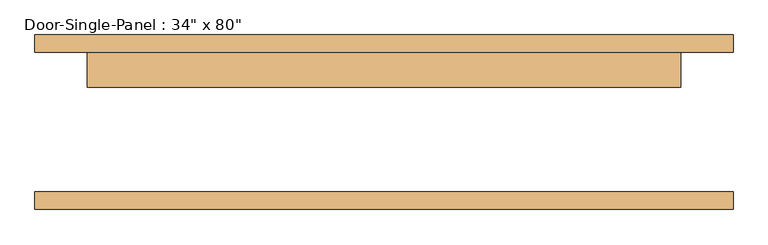
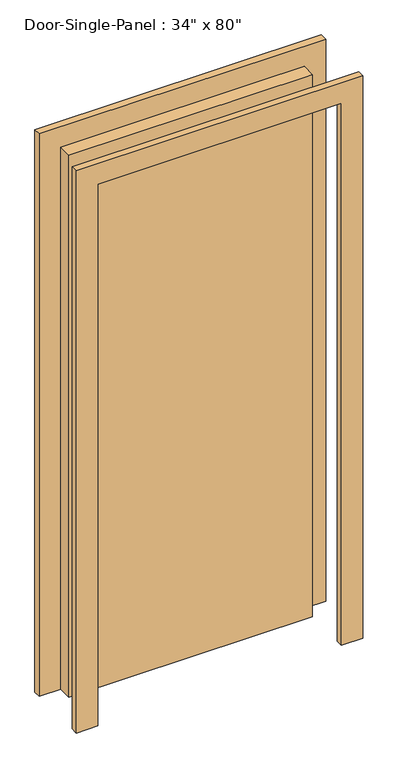
"""IFC4 building model written with IfcOpenShell, lengths in millimetres: door geometry."""

from ifc_helpers import new_model, si_unit, frame, origin, origin_with_axes, place, context, project, spatial, polyline, outline, extrude, source, transform, mapped, element, save


def door_10fd3a06(model_context):
    return source(origin(), model_context, "Body", "SweptSolid", [
        extrude(outline(polyline([(431.8, 50.8), (-431.8, 50.8), (-431.8, 101.6), (431.8, 101.6), (431.8, 50.8)])), origin_with_axes(), (0.0, 0.0, 1.0), 2032.0),
        extrude(outline(polyline([(2108.2, -508.0), (0.0, -508.0), (0.0, -431.8), (2032.0, -431.8), (2032.0, 431.8), (0.0, 431.8), (0.0, 508.0), (2108.2, 508.0), (2108.2, -508.0)])), frame((0.0, 101.6, 0.0), z_axis=(0.0, 1.0, 0.0), x_axis=(0.0, 0.0, 1.0)), (0.0, 0.0, 1.0), 25.4),
        extrude(outline(polyline([(2108.2, 508.0), (2108.2, -508.0), (0.0, -508.0), (0.0, -431.8), (2032.0, -431.8), (2032.0, 431.8), (0.0, 431.8), (0.0, 508.0), (2108.2, 508.0)])), frame((0.0, -127.0, 0.0), z_axis=(0.0, 1.0, 0.0), x_axis=(0.0, 0.0, 1.0)), (0.0, 0.0, 1.0), 25.4),
    ])


if __name__ == "__main__":
    model = new_model("IFC4")
    model_context = context("Model", 3, world=origin())
    ifc_project = project(units=[si_unit("LENGTHUNIT", "METRE", prefix="MILLI")], contexts=[model_context])
    site = spatial("IfcSite", under=ifc_project)
    building = spatial("IfcBuilding", under=site)
    placement = place(None, origin())
    door_shape = door_10fd3a06(model_context)
    element("IfcDoor", 1, ObjectType="Door-Single-Panel : 34\" x 80\"", at=placement, inside=building, context=model_context, shape_type="MappedRepresentation", body=[
        mapped(door_shape, transform((0.0, 0.0, 0.0), x_axis=(1.0, 0.0, 0.0), y_axis=(0.0, 1.0, 0.0), z_axis=(0.0, 0.0, 1.0))),
    ])
    save(model, "model.ifc")

# Revit data of these elements
# Type "Door-Single-Panel : 34\" x 80\""
#   Type Mark = "8"
#   Construction Type Id = "DOOR"
#   Assembly Code = "C1020300"
#   Analytic Construction = "Wooden"
#   Thickness = 0' - 2"
#   Thermal Resistance (R) = 2.5876 (h·ft²·°F)/BTU
#   Swing Angle [instance default] = 90.00°
#   Heat Transfer Coefficient (U) = 0.3865 BTU/(h·ft²·°F)
#   Height = 6' - 8"
#   Trim Projection Ext = 0' - 1"
#   Trim Projection Int = 0' - 1"
#   Trim Width = 0' - 3"
#   Width = 2' - 10"
#   Define Thermal Properties by = 1
#   Panel Material = Wood - Birch - Solid Stained Light Low Gloss
#   Trim Material = Paint - Sienna
#   Visual Light Transmittance = 0
#   Solar Heat Gain Coefficient = 0
#   Function = (empty or 0)
#   Wall Closure = (empty or 0)
# Element 1 (IfcDoor, "Door-Single-Panel : 34\" x 80\"")
#   Materials on its faces: "Paint - Sienna", "Wood - Birch - Solid Stained Light Low Gloss"
# Materials
#   "Wood - Birch - Solid Stained Light Low Gloss": class "Wood", colour RGB 210 159 95, transparency 0, Cost = 0
#   "Paint - Sienna": colour RGB 118 70 51, transparency 0, Cost = 0
